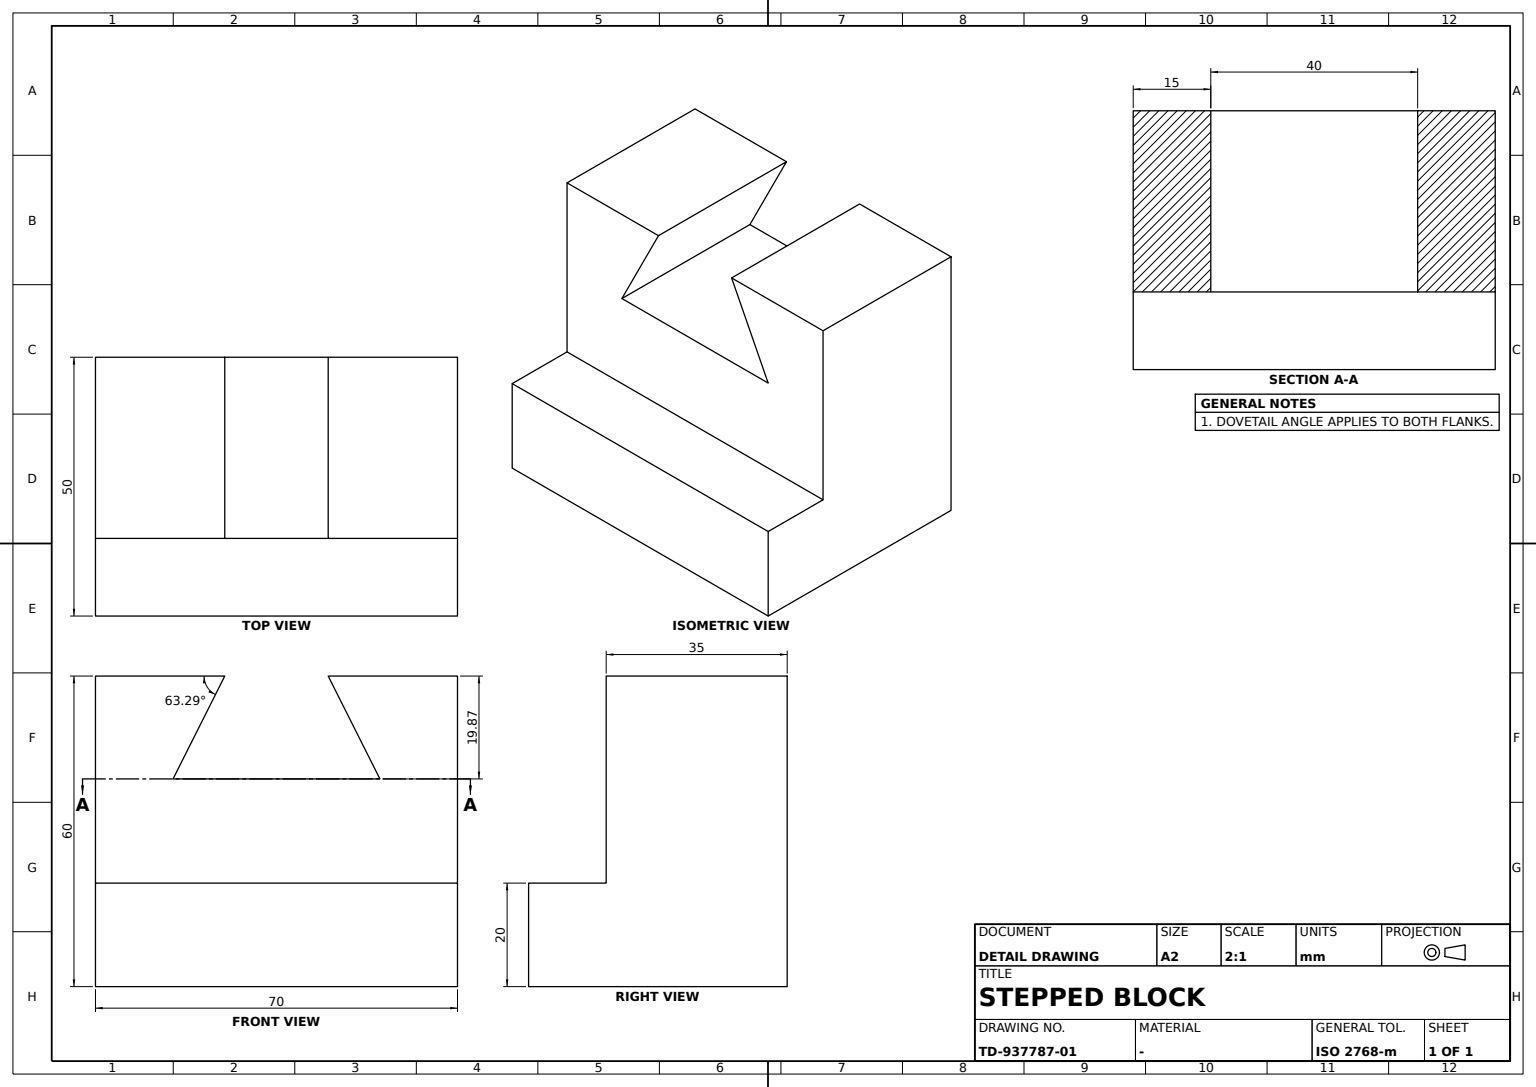
CATIA V5 part; units mm, degrees
sketch "Sketch1" plane through (0, 0, 0) normal (1, 0, 0) x (0, 1, 0)
  line L0 (0, 0) -> (50, 0)
  line L1 (50, 0) -> (50, 20)
  line L2 (50, 20) -> (35, 20)
  line L3 (35, 20) -> (35, 60)
  line L4 (35, 60) -> (0, 60)
  point P0 (0, 60)
  line L5 (0, 60) -> (0, 0)
  dimension "length L1" = 20
  dimension "length L0" = 50
  dimension "length L4" = 35
  dimension "length L5" = 60
  constraint horizontal L0 x-axis
  constraint horizontal L2 x-axis
  constraint horizontal L4 x-axis
  constraint vertical L1 y-axis
  constraint vertical L3 y-axis
  constraint vertical L5 y-axis
  constraint coincidence P0 y-axis
extrude "Pad1" add sketch "Sketch1" along normal mid plane 70
sketch "Sketch2" plane through (0, 35, 0) normal (0, 1, 0) x (-1, 0, 0)
  line L0 (-20, 40.1275) -> (20, 40.1275)
  point P0 (20, 40.1275)
  line L1 (35, 20) -> (35, 60) construction
  line L2 (-20, 40.1275) -> (-10, 60)
  line L3 (-10, 60) -> (10, 60)
  line L4 (10, 60) -> (20, 40.1275)
  dimension "length L0" = 40
  dimension "distance P0 L1" = 15
  constraint horizontal L0 x-axis
  constraint horizontal L3 x-axis
extrude "Pocket1" cut sketch "Sketch2" against normal up to next
properties part number "catia 5"
